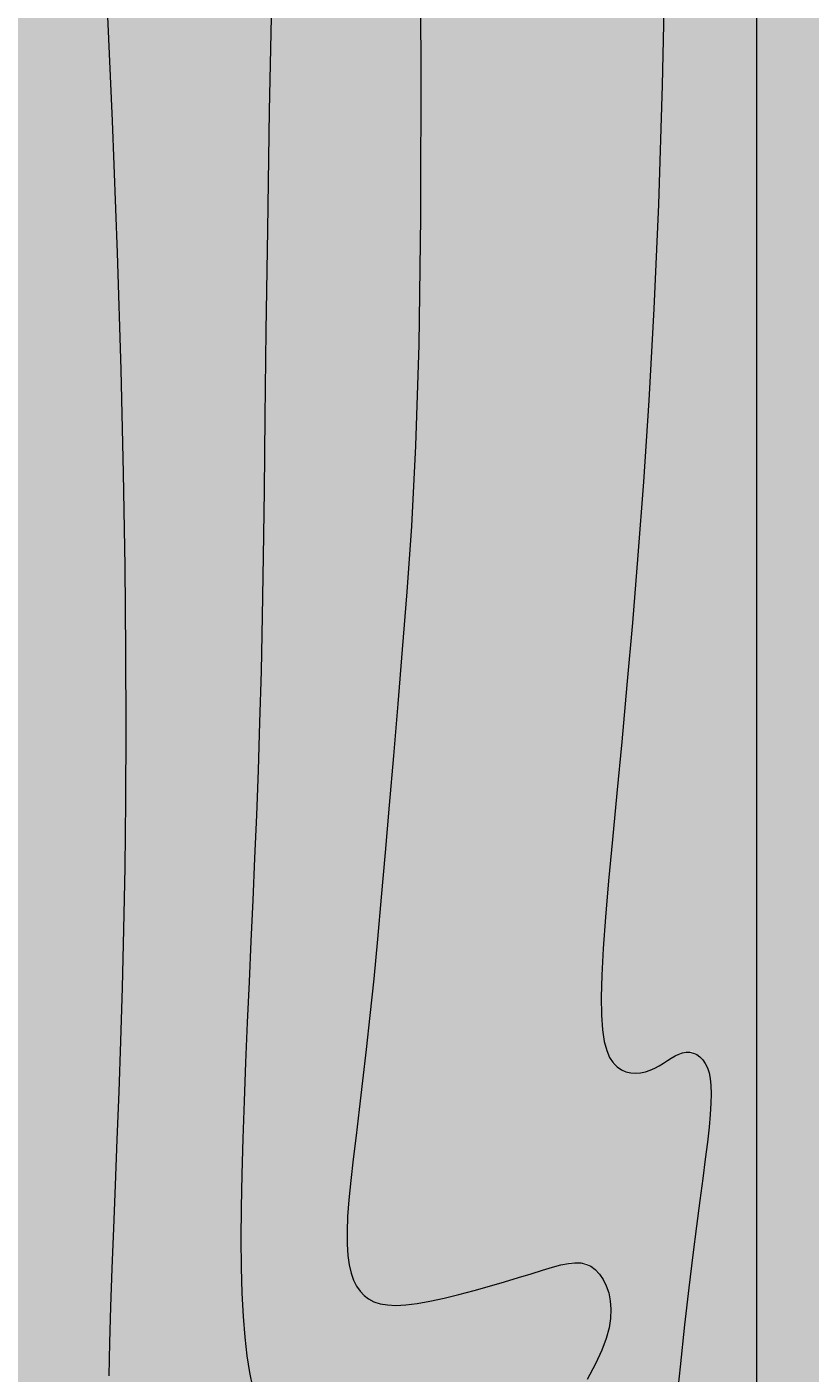
# Model space of a CAD drawing. Units: millimetres. Extents: x -229 to 16545, y -10488 to 4272.
# Tile 17 of 29: x 12216 to 12629, y -3417 to -2708. Entities that reach past the tile are written whole.
import ezdxf

# ---------------------------------------------------------------- set-up
doc = ezdxf.new("R2010")
doc.units = ezdxf.units.MM
for name, color, linetype, lineweight in [('A-ANNO-DIMS', 2, 'Continuous', 18), ('A-FURN', 8, 'Continuous', 18), ('A-FURN-PATT', 252, 'Continuous', 13)]:
    doc.layers.add(name, color=color, linetype=linetype, lineweight=lineweight)
doc.layers.add('A-FLOR-PATT', color=254, linetype='Continuous', lineweight=13, true_color=0xfeeab9)
doc.styles.get("Standard").update_dxf_attribs({"font": 'arial.ttf'})
doc.dimstyles.get("Standard").update_dxf_attribs({"dimtxt": 0.18, "dimasz": 0.18, "dimexe": 0.18, "dimexo": 0.0625, "dimgap": 0.09, "dimtad": 0, "dimtih": 1, "dimtoh": 1, "dimdec": 4, "dimzin": 0, "dimdsep": 46, "dimtxsty": 'Standard', "dimcen": 0.09, "dimadec": 0, "dimazin": 0, "dimtfac": 1, "dimtdec": 4, "dimtofl": 0, "dimtmove": 0, "dimatfit": 3, "dimfxl": 1, "dimtolj": 1, "dimtzin": 0, "dimarcsym": 0})

# ---------------------------------------------------------------- blocks, each defined once
blk = doc.blocks.new('Table - Rectangular Woodgrain 60 x 30 in.')
blk.add_line((60, 0), (0, 0))
for points in [[(9.0302, -2.4688), (12.709, -2.5477), (15.9167, -2.65), (18.7181, -2.7711), (21.1781, -2.9063), (23.3616, -3.0508), (25.3333, -3.2), (27.1477, -3.3495), (28.8172, -3.4958), (30.3437, -3.636), (31.7291, -3.7667), (32.9756, -3.8849), (34.0849, -3.9875), (35.059, -4.0714), (35.9, -4.1334), (36.6114, -4.1711), (37.2041, -4.1854), (37.6906, -4.1779), (38.0833, -4.15), (38.3948, -4.1034), (38.6375, -4.0396), (38.8239, -3.9602), (38.9666, -3.8667), (39.0764, -3.7608), (39.1573, -3.6448), (39.2116, -3.521), (39.2416, -3.3917), (39.2498, -3.2593), (39.2385, -3.1261), (39.21, -2.9944), (39.1666, -2.8667), (39.111, -2.7447), (39.0468, -2.6281), (38.978, -2.5163), (38.9083, -2.4083), (38.8418, -2.3035), (38.7823, -2.201), (38.7337, -2.1001), (38.7, -2), (38.6844, -1.9003), (38.6875, -1.8021), (38.7094, -1.707), (38.75, -1.6167), (38.8094, -1.5326), (38.8875, -1.4563), (38.9844, -1.3893), (39.1, -1.3333), (39.2351, -1.2896), (39.3937, -1.2583), (39.5804, -1.2396), (39.8, -1.2333), (40.057, -1.2396), (40.3562, -1.2583), (40.7023, -1.2896), (41.1, -1.3333), (41.5547, -1.3895), (42.0755, -1.4573), (42.6721, -1.5361), (43.3542, -1.625), (44.1316, -1.7233), (45.014, -1.8302), (46.0114, -1.9449), (47.1333, -2.0667), (48.3862, -2.1947)], [(6.5759, -9.0858), (11.9385, -9.0365), (16.2527, -9.0418), (19.6833, -9.0917), (22.3952, -9.1759), (24.5531, -9.2844), (26.322, -9.4069), (27.8666, -9.5333), (29.3241, -9.6553), (30.7203, -9.7719), (32.0532, -9.8837), (33.3208, -9.9917), (34.5213, -10.0965), (35.6526, -10.199), (36.7128, -10.2999), (37.7, -10.4), (38.6129, -10.4996), (39.4531, -10.5969), (40.223, -10.6895), (40.925, -10.775), (41.5613, -10.8512), (42.1344, -10.9156), (42.6465, -10.966), (43.1, -11), (43.4976, -11.0158), (43.8437, -11.0136), (44.143, -10.9942), (44.4, -10.9583), (44.6195, -10.9069), (44.8062, -10.8406), (44.9648, -10.7603), (45.1, -10.6667), (45.2155, -10.5598), (45.3114, -10.4365), (45.3871, -10.2929), (45.4416, -10.125), (45.4743, -9.929), (45.4844, -9.7011), (45.4709, -9.4371), (45.4333, -9.1333), (45.3716, -8.7883), (45.2896, -8.4104), (45.1919, -8.0107), (45.0833, -7.6), (44.9685, -7.1893), (44.8521, -6.7896), (44.7388, -6.4117), (44.6333, -6.0667), (44.54, -5.7628), (44.4614, -5.4979), (44.4001, -5.2675), (44.3583, -5.0667), (44.3384, -4.8909), (44.3427, -4.7354), (44.3736, -4.5956), (44.4333, -4.4667), (44.5236, -4.3453), (44.6427, -4.2333), (44.7884, -4.1339), (44.9583, -4.05), (45.1501, -3.9849), (45.3614, -3.9417), (45.59, -3.9234), (45.8333, -3.9333), (46.0915, -3.9749), (46.3734, -4.0531), (46.6906, -4.1736), (47.0542, -4.3417), (47.4756, -4.5629)], [(9.6213, -13.0323), (13.3963, -13.1059), (16.5958, -13.1583), (19.3063, -13.1952), (21.614, -13.2219), (23.6054, -13.2439), (25.3666, -13.2667), (26.9728, -13.2947), (28.4531, -13.3281), (29.8256, -13.3663), (31.1083, -13.4083), (32.3191, -13.4535), (33.476, -13.501), (34.597, -13.5501), (35.7, -13.6), (36.7984, -13.6497), (37.8875, -13.6979), (38.9578, -13.743), (40, -13.7833), (41.0047, -13.8174), (41.9625, -13.8438), (42.864, -13.8607), (43.7, -13.8667), (44.4631, -13.8604), (45.1552, -13.8417), (45.7801, -13.8104), (46.3416, -13.7667), (46.8439, -13.7104), (47.2906, -13.6417), (47.6858, -13.5604)], [(9.6609, -17.5057), (13.6705, -17.3303), (17.2125, -17.1958), (20.3467, -17.0973), (23.1328, -17.0297), (25.6307, -16.9878), (27.9, -16.9667), (29.9928, -16.9617), (31.9302, -16.9703), (33.7254, -16.9907), (35.3917, -17.0208), (36.9423, -17.0588), (38.3906, -17.1026), (39.7499, -17.1503), (41.0333, -17.2), (42.2519, -17.2496), (43.4073, -17.2969), (44.4986, -17.3395), (45.525, -17.375), (46.4858, -17.4012), (47.3802, -17.4156)]]:
    blk.add_lwpolyline(points)
blk = doc.blocks.new('*D101')
at = {"layer": 'A-ANNO-DIMS', "color": 0, "lineweight": -2, "transparency": 16777216}
for p, q in [((10907.81, -3049.71), (10907.99, -3049.71)), ((10907.9, -3049.8), (10907.9, -3049.62)), ((15176.85, -3049.71), (13576.18, -3049.71))]:
    blk.add_line(p, q, dxfattribs=at)
at = {"layer": 'A-ANNO-DIMS', "color": 0, "transparency": 16777216}
blk.add_solid([(13576.18, -3049.68), (13576.18, -3049.74), (13576, -3049.71)], dxfattribs=at)
at = {"layer": 'Defpoints', "color": 0, "transparency": 16777216}
for p in [(10907.9, -3049.71), (13576, -3049.71)]:
    blk.add_point(p, dxfattribs=at)
at = {"layer": 'A-ANNO-DIMS', "color": 0, "transparency": 16777216, "insert": (15177.3, -3049.71), "char_height": 0.18, "attachment_point": 5}
blk.add_mtext('\\A1;R2668', dxfattribs=at)
blk = doc.blocks.new('*D102')
at = {"layer": 'A-ANNO-DIMS', "color": 0, "lineweight": -2, "transparency": 16777216}
for p, q in [((11192.83, -3049.71), (11193.01, -3049.71)), ((11192.92, -3049.8), (11192.92, -3049.62)), ((15217.18, -3049.71), (13708.26, -3049.71))]:
    blk.add_line(p, q, dxfattribs=at)
at = {"layer": 'A-ANNO-DIMS', "color": 0, "transparency": 16777216}
blk.add_solid([(13708.26, -3049.68), (13708.26, -3049.74), (13708.08, -3049.71)], dxfattribs=at)
at = {"layer": 'Defpoints', "color": 0, "transparency": 16777216}
for p in [(11192.92, -3049.71), (13708.08, -3049.71)]:
    blk.add_point(p, dxfattribs=at)
at = {"layer": 'A-ANNO-DIMS', "color": 0, "transparency": 16777216, "insert": (15217.62, -3049.71), "char_height": 0.18, "attachment_point": 5}
blk.add_mtext('\\A1;R2515', dxfattribs=at)

msp = doc.modelspace()

# ---------------------------------------------------------------- hatches: boundary and pattern name
at = {"layer": 'A-FLOR-PATT', "transparency": 33554592}
h = msp.add_hatch(color=256, dxfattribs=at)
h.dxf.hatch_style = 1
h.paths.add_polyline_path([(7975.933, -5325.772), (7943.121, -5325.772), (7943.121, -4576.49, 0.4014527), (7225.933, -5325.772, 0.4014527), (6508.746, -4576.49), (6508.746, -5325.772), (6475.933, -5325.772), (6475.933, -5438.272), (5975.933, -5438.272), (5975.933, -7267.724), (5975.933, -7438.272), (6478.619, -7438.272), (6463.448, -7355.919), (6464.88, -7356.837), (6463.849, -7358.097), (6478.619, -7438.272), (6610.327, -7438.272), (6632.656, -7409.564), (6632.525, -7406.967), (6634.208, -7407.569), (6619.273, -7426.77), (6654.466, -7438.272), (7610.517, -7438.272), (7607.41, -7421.409), (7608.842, -7422.327), (7607.812, -7423.587), (7610.517, -7438.272), (7975.933, -7438.272)])
h.paths.add_polyline_path([(13785.933, -1208.272), (9555.933, -1208.272), (9555.933, -961.785), (9705.933, -961.785), (9705.933, -918.035), (10704.976, -918.035, 0.4014527), (9705.933, 38.215), (9555.933, 38.215), (9555.933, 2021.728), (5975.933, 2021.728), (5975.933, 755.492), (5745.933, 755.492), (5745.933, 1427.266), (2918.813, 1427.266), (2918.813, -492.942), (5013.319, -492.942), (5013.319, -978.272), (5745.933, -978.272), (5745.933, -397.513), (5975.933, -397.513), (5975.933, -1208.272), (4560.933, -1208.272), (4560.933, -1265.772), (4448.433, -1265.772), (4448.433, -1298.585), (4445.933, -1298.585), (3699.151, -1298.585, 0.4014527), (4448.433, -2015.772), (4560.933, -2015.772), (4560.933, -2384.177), (5745.933, -2384.177), (5799.402, -2384.177), (5799.402, -4518.272), (5975.933, -4518.272), (5975.933, -5208.272), (6475.933, -5208.272), (6475.933, -4575.772), (6508.746, -4575.772), (6508.746, -4576.49, -0.3564726), (7216.672, -5208.272), (7235.194, -5208.272, -0.3564726), (7943.121, -4576.49), (7943.121, -4575.772), (7975.933, -4575.772), (7975.933, -5208.272), (11176.247, -5208.272), (11159.44, -5191.465), (10520.768, -5191.465), (10520.768, -4888.936), (10571.19, -4888.936), (10571.19, -4872.129), (10772.876, -4872.129), (10772.876, -4888.936), (10789.683, -4888.936), (10789.683, -4872.129), (10991.368, -4872.129), (10991.368, -4888.936), (11041.79, -4888.936), (11041.79, -4872.129), (11058.597, -4872.129, -0.0909091), (11428.354, -4872.129), (11445.162, -4872.129), (11445.162, -4888.936), (11529.197, -4888.936), (11529.197, -5191.465), (11327.512, -5191.465), (11310.704, -5208.272), (13785.933, -5208.272)])
h.paths.add_polyline_path([(11047.216, -1630.944, -1), (11402.816, -1630.944, -1)], flags=16)
h.paths.add_polyline_path([(11148.816, -1630.944), (11225.016, -1554.744), (11301.216, -1630.944), (11225.016, -1707.144)], flags=0)
h.paths.add_polyline_path([(11199.616, -1630.944, -1), (11250.416, -1630.944, -1)], flags=0)
h.paths.add_polyline_path([(11588.751, -2096.259), (11588.751, -1543.254, -0.266667), (12864.918, -1543.254), (12864.918, -2096.259), (12737.302, -2096.259), (12737.302, -2063.121), (11716.368, -2063.121), (11716.368, -2096.259)], flags=16)
h.paths.add_polyline_path([(12012.696, -2489.42), (12600.997, -2489.42), (12600.997, -3666.022), (12012.696, -3666.022)], flags=16)
h.paths.add_polyline_path([(12176.41, -3599.403), (12174.938, -3609.076), (12173.789, -3618.819), (12173.09, -3628.559), (12172.973, -3638.221), (12173.89, -3652.852), (12175.008, -3657.025), (12172.909, -3643.473), (12173.142, -3624.297), (12175.386, -3605.273)], flags=0)
h.paths.add_polyline_path([(8026.289, -286.944), (7737.703, -287.19), (7734.87, -269.156), (8029.092, -268.905)], flags=16)
h.paths.add_polyline_path([(7733.453, -260.139), (7710.784, -115.865), (7557.191, -115.996), (7556.999, 109.744), (7412.687, 132.166), (7412.433, 429.206), (7556.707, 451.876), (7556.568, 614.769), (7412.256, 637.19), (7412.003, 934.231), (7556.276, 956.9), (7556.084, 1182.639), (7709.677, 1182.77), (7732.099, 1327.082), (8029.14, 1327.335), (8051.808, 1183.062), (8205.401, 1183.192), (8205.594, 957.454), (8349.906, 935.031), (8350.159, 637.99), (8205.885, 615.322), (8206.024, 452.43), (8350.336, 430.006), (8350.59, 132.965), (8206.316, 110.298), (8206.509, -115.442), (8052.916, -115.573), (8030.493, -259.885)], flags=16)
h.paths.add_polyline_path([(12261.416, -3475.554), (12262.632, -3486.776), (12264.032, -3497.007), (12265.554, -3506.365), (12267.136, -3514.968), (12268.719, -3522.935), (12271.304, -3535.59), (12273.606, -3548.078), (12275.271, -3561.064), (12275.93, -3574.938), (12275.325, -3590.3), (12273.425, -3607.964), (12270.795, -3625.658), (12268.066, -3641.063), (12266.318, -3649.679), (12265.456, -3653.626), (12263.984, -3659.846), (12264.032, -3659.566), (12264.342, -3658.241), (12264.807, -3656.37), (12265.456, -3653.626), (12266.318, -3649.679), (12267.409, -3644.302), (12268.668, -3637.664), (12270.019, -3630.037), (12271.384, -3621.695), (12272.69, -3612.908), (12273.857, -3603.948), (12274.81, -3595.088), (12275.47, -3586.601), (12275.782, -3578.689), (12275.757, -3571.292), (12275.423, -3564.275), (12274.816, -3557.512), (12273.964, -3550.872), (12272.896, -3544.224), (12271.645, -3537.439), (12270.24, -3530.385), (12267.543, -3517.181), (12264.612, -3501.247), (12261.849, -3481.059)], flags=0)
h.paths.add_polyline_path([(12332.136, -3408.03), (12333.483, -3416.79), (12335.077, -3424.54), (12336.915, -3431.355), (12338.991, -3437.32), (12341.266, -3442.55), (12343.694, -3447.166), (12346.229, -3451.292), (12348.826, -3455.051), (12351.438, -3458.563), (12357.476, -3466.491), (12363.61, -3476.575), (12368.309, -3489.762), (12369.929, -3503.427), (12369.842, -3516.511), (12368.43, -3530.867), (12365.816, -3545.835), (12362.382, -3559.786), (12360.968, -3564.487), (12363.063, -3557.021), (12364.898, -3549.566), (12366.473, -3542.077), (12367.773, -3534.631), (12368.781, -3527.301), (12369.483, -3520.162), (12369.863, -3513.291), (12369.906, -3506.759), (12369.599, -3500.643), (12368.93, -3494.999), (12367.924, -3489.796), (12366.61, -3484.994), (12365.024, -3480.542), (12363.19, -3476.399), (12361.141, -3472.516), (12358.909, -3468.847), (12356.525, -3465.347), (12354.02, -3461.954), (12351.438, -3458.563), (12345.462, -3450.529), (12339.923, -3439.996), (12335.85, -3428.296), (12332.68, -3412.888)], flags=0)
h.paths.add_polyline_path([(12385.287, -3334.612), (12384.977, -3342.409), (12385.02, -3349.196), (12385.4, -3355.066), (12386.104, -3360.105), (12387.112, -3364.41), (12388.412, -3368.071), (12389.987, -3371.181), (12391.823, -3373.832), (12393.919, -3376.097), (12396.337, -3377.978), (12399.153, -3379.462), (12402.445, -3380.531), (12406.289, -3381.172), (12410.758, -3381.371), (12415.935, -3381.106), (12421.893, -3380.368), (12428.658, -3379.159), (12436.069, -3377.55), (12443.907, -3375.635), (12451.961, -3373.505), (12460.015, -3371.254), (12467.853, -3368.971), (12475.263, -3366.749), (12482.029, -3364.68), (12491.877, -3361.657), (12497.701, -3360.107), (12501.639, -3359.288), (12510.135, -3358.326), (12519.662, -3365.412), (12524.243, -3378.911), (12523.764, -3390.7), (12520.746, -3401.577), (12514.248, -3415.634), (12511.518, -3420.418), (12515.856, -3412.154), (12519.153, -3405.024), (12521.516, -3398.804), (12523.049, -3393.276), (12523.865, -3388.212), (12524.059, -3383.441), (12523.7, -3378.958), (12522.853, -3374.815), (12521.576, -3371.054), (12519.931, -3367.722), (12517.982, -3364.865), (12515.786, -3362.529), (12513.405, -3360.758), (12510.877, -3359.588), (12508.136, -3358.982), (12505.086, -3358.897), (12501.639, -3359.288), (12497.701, -3360.107), (12493.183, -3361.309), (12487.988, -3362.851), (12476.403, -3366.408), (12463.335, -3370.326), (12447.372, -3374.788), (12431.759, -3378.604), (12418.504, -3380.974), (12405.811, -3381.624), (12394.725, -3378.025), (12388.039, -3368.367), (12385.583, -3357.877), (12384.826, -3346.204), (12385.428, -3331.059), (12385.953, -3325.719)], flags=0)
h.paths.add_polyline_path([(7880.016, 1173.969), (7880.373, 1175.495), (7880.433, 1175.851), (7879.484, 1171.818)], flags=0)
h.paths.add_polyline_path([(7802.33, 874.962), (7800.771, 885.032), (7798.932, 893.941), (7796.811, 901.774), (7794.419, 908.63), (7791.798, 914.639), (7789.002, 919.945), (7786.083, 924.686), (7783.093, 929.005), (7780.087, 933.043), (7774.996, 939.717), (7768.406, 949.37), (7762.174, 963.427), (7759.342, 978.002), (7758.629, 991.888), (7759.492, 1007.928), (7761.801, 1025.496), (7765.392, 1044.035), (7766.625, 1049.048), (7764.522, 1039.543), (7762.719, 1030.232), (7761.232, 1021.168), (7760.08, 1012.405), (7759.28, 1003.994), (7758.849, 995.988), (7758.806, 988.44), (7759.167, 981.404), (7759.942, 974.914), (7761.104, 968.936), (7762.617, 963.414), (7764.448, 958.299), (7766.559, 953.535), (7768.918, 949.073), (7771.487, 944.856), (7774.232, 940.835), (7777.115, 936.938), (7782.377, 930.041), (7787.845, 922.139), (7793.348, 911.698), (7798.042, 898.247), (7801.702, 880.527)], flags=0)
h.paths.add_polyline_path([(12519.068, -3228.534), (12519.615, -3236.235), (12520.529, -3242.343), (12521.78, -3247.103), (12523.337, -3250.758), (12525.171, -3253.556), (12527.248, -3255.709), (12529.522, -3257.296), (12531.95, -3258.361), (12534.486, -3258.949), (12537.082, -3259.11), (12539.694, -3258.888), (12542.277, -3258.329), (12544.781, -3257.478), (12547.173, -3256.388), (12549.46, -3255.129), (12550.455, -3254.517), (12555.825, -3251.109), (12557.835, -3249.942), (12565.181, -3246.404), (12574.565, -3253.032), (12576.931, -3265.022), (12576.627, -3277.425), (12575.416, -3290.819), (12574.851, -3295.392), (12575.708, -3287.593), (12576.322, -3280.806), (12576.688, -3274.939), (12576.812, -3269.899), (12576.688, -3265.593), (12576.322, -3261.932), (12575.708, -3258.822), (12574.851, -3256.172), (12573.753, -3253.905), (12572.439, -3252.005), (12570.943, -3250.474), (12569.293, -3249.309), (12567.523, -3248.513), (12565.658, -3248.083), (12563.732, -3248.022), (12561.777, -3248.328), (12559.814, -3248.989), (12557.835, -3249.942), (12555.825, -3251.109), (12553.77, -3252.413), (12551.652, -3253.78), (12549.46, -3255.129), (12543.167, -3258.594), (12532.661, -3259.485), (12524.685, -3253.923), (12520.949, -3245.152), (12519.138, -3233.042)], flags=0)
h.paths.add_polyline_path([(7741.293, 790.501), (7741.641, 799.467), (7741.584, 807.269), (7741.141, 814.015), (7740.329, 819.809), (7739.165, 824.757), (7737.667, 828.966), (7735.853, 832.541), (7733.74, 835.586), (7731.348, 838.188), (7728.71, 840.348), (7725.861, 842.052), (7722.836, 843.28), (7719.671, 844.015), (7716.4, 844.237), (7713.06, 843.932), (7709.684, 843.081), (7706.304, 841.686), (7702.923, 839.834), (7699.543, 837.629), (7696.164, 835.178), (7692.784, 832.585), (7684.718, 826.315), (7675.609, 820.63), (7664.001, 817.274), (7654.105, 821.884), (7647.171, 832.02), (7644.191, 846.522), (7646.321, 860.288), (7647.49, 864.223), (7645.946, 857.865), (7645.046, 852.044), (7644.827, 846.557), (7645.243, 841.404), (7646.221, 836.642), (7647.693, 832.318), (7649.587, 828.489), (7651.832, 825.206), (7654.359, 822.523), (7657.097, 820.49), (7659.984, 819.145), (7662.993, 818.452), (7666.108, 818.357), (7669.311, 818.809), (7672.583, 819.755), (7675.908, 821.139), (7679.268, 822.913), (7682.645, 825.021), (7686.025, 827.401), (7689.404, 829.958), (7692.784, 832.585), (7700.505, 838.509), (7709.871, 843.64), (7721.436, 844.698), (7733.277, 837.617), (7739.571, 825.214), (7741.557, 811.049), (7741.669, 795.575)], flags=0)
h.paths.add_polyline_path([(8377.641, 137.216), (8359.607, 134.382), (8359.356, 428.605), (8377.395, 425.802)], flags=16)
h.paths.add_polyline_path([(7650.715, 668.465), (7650.08, 677.319), (7649.023, 684.34), (7647.579, 689.811), (7645.785, 694.012), (7643.675, 697.228), (7641.286, 699.7), (7638.669, 701.521), (7635.876, 702.744), (7632.96, 703.419), (7629.974, 703.601), (7626.971, 703.344), (7624.004, 702.697), (7621.125, 701.717), (7618.375, 700.462), (7615.749, 699.013), (7614.561, 698.279), (7608.435, 694.382), (7606.125, 693.04), (7598.981, 689.594), (7589.669, 693.773), (7585.26, 702.856), (7584.221, 713.11), (7584.49, 724.584), (7585.863, 739.937), (7586.518, 745.277), (7585.539, 736.31), (7584.841, 728.507), (7584.424, 721.761), (7584.288, 715.966), (7584.433, 711.016), (7584.86, 706.807), (7585.567, 703.231), (7586.556, 700.186), (7587.821, 697.58), (7589.332, 695.397), (7591.053, 693.637), (7592.951, 692.3), (7594.989, 691.385), (7597.132, 690.895), (7599.346, 690.826), (7601.594, 691.18), (7603.851, 691.943), (7606.125, 693.04), (7608.435, 694.382), (7610.797, 695.885), (7613.229, 697.458), (7620.475, 701.929), (7632.001, 704.44), (7643.476, 699.417), (7648.536, 687.571), (7650.63, 673.661)], flags=0)
h.paths.add_polyline_path([(7385.628, 136.37), (7385.382, 424.956), (7403.416, 427.789), (7403.667, 133.567)], flags=16)
h.paths.add_polyline_path([(12993.884, -2257.186), (12959.588, -2257.186), (12959.588, -2125.099), (13531.966, -2125.099, -0.1904762), (13531.966, -3974.321), (12959.588, -3974.321), (12959.588, -3842.233), (12993.884, -3842.233)], flags=16)
h.paths.add_polyline_path([(13413.486, -3313.884), (13413.486, -2785.535), (13562.885, -2785.535, -0.0496282), (13562.885, -3313.884)], flags=0)
h.paths.add_polyline_path([(8377.21, 642.241), (8359.176, 639.407), (8358.925, 933.629), (8376.964, 930.826)], flags=16)
h.paths.add_polyline_path([(13086.058, -1864.83), (13086.058, -1449.84), (13501.048, -1449.84), (13501.048, -1864.83)], flags=16)
h.paths.add_polyline_path([(13305.814, -1862.197), (13302.103, -1859.624), (13298.088, -1857.068), (13293.799, -1854.536), (13289.262, -1852.031), (13284.504, -1849.559), (13279.554, -1847.125), (13274.439, -1844.735), (13269.17, -1842.389), (13263.701, -1840.081), (13257.97, -1837.797), (13251.914, -1835.525), (13245.472, -1833.252), (13238.582, -1830.968), (13231.18, -1828.66), (13223.206, -1826.315), (13209.182, -1822.458), (13204.584, -1821.48), (13217.962, -1824.773), (13235.072, -1829.804), (13248.777, -1834.349), (13260.829, -1838.869), (13274.479, -1844.63), (13289.675, -1852.101), (13302.553, -1859.704)], flags=0)
h.paths.add_polyline_path([(13428.104, -1820.994), (13419.007, -1818.141), (13409.95, -1815.4), (13400.766, -1812.747), (13391.271, -1810.151), (13376.087, -1806.251), (13370.618, -1805.019), (13386.304, -1808.794), (13405.087, -1813.928), (13423.014, -1819.354)], flags=0)
h.paths.add_polyline_path([(7385.197, 641.395), (7384.951, 929.98), (7402.986, 932.814), (7403.236, 638.592)], flags=16)
h.paths.add_polyline_path([(13262.537, -1725.526), (13253.246, -1724.74), (13244.516, -1724.117), (13235.94, -1723.625), (13223.267, -1723.062), (13217.598, -1722.912), (13231.966, -1723.397), (13248.733, -1724.359), (13266.899, -1725.895), (13272.802, -1726.502)], flags=0)
h.paths.add_polyline_path([(13191.893, -1641.137), (13208.675, -1640.506), (13214.057, -1640.258), (13197.763, -1640.936)], flags=0)
h.paths.add_polyline_path([(13097.524, -1608.457), (13114.284, -1609.031), (13120.126, -1609.105), (13103.045, -1608.71)], flags=0)
h.paths.add_polyline_path([(13465.328, -1521.577), (13473.906, -1517.015), (13481.761, -1511.636), (13492.562, -1502.076), (13495.327, -1497.933), (13485.818, -1508.858), (13470.208, -1519.547)], flags=0)
h.paths.add_polyline_path([(13175.015, -1500.891), (13184.046, -1501.807), (13192.721, -1502.52), (13201.114, -1503.034), (13209.273, -1503.351), (13217.244, -1503.476), (13225.078, -1503.41), (13232.821, -1503.16), (13240.524, -1502.728), (13248.233, -1502.117), (13255.993, -1501.322), (13263.825, -1500.293), (13271.746, -1498.974), (13279.775, -1497.305), (13287.928, -1495.229), (13296.222, -1492.688), (13304.675, -1489.622), (13313.304, -1485.975), (13322.089, -1481.727), (13330.859, -1477.028), (13339.408, -1472.063), (13347.526, -1467.02), (13355.006, -1462.087), (13364.86, -1455.202), (13367.224, -1453.299), (13358.544, -1459.754), (13343.348, -1469.775), (13326.143, -1479.767), (13309.023, -1488.045), (13292.249, -1494.129), (13276.009, -1498.264), (13260.299, -1500.88), (13244.401, -1502.51), (13228.945, -1503.378), (13213.316, -1503.508), (13197.047, -1502.876), (13180.088, -1501.481)], flags=0)
h.paths.add_polyline_path([(7733.501, 1336.101), (7736.303, 1354.14), (8024.889, 1354.386), (8027.723, 1336.352)], flags=16)
at = {"layer": 'A-FURN-PATT', "transparency": 33554569}
h = msp.add_hatch(color=256, dxfattribs=at)
h.dxf.hatch_style = 1
h.paths.add_polyline_path([(12600.997, -2489.42), (12553.933, -2489.42), (12553.58, -2583.852), (12552.584, -2666.503), (12551.036, -2738.644), (12549.03, -2801.547), (12546.656, -2856.483), (12544.004, -2904.723), (12541.171, -2947.542), (12538.245, -2986.207), (12535.313, -3021.787), (12532.444, -3054.526), (12529.695, -3084.461), (12527.132, -3111.629), (12524.814, -3136.073), (12522.802, -3157.826), (12521.157, -3176.928), (12519.941, -3193.42), (12519.202, -3207.371), (12518.921, -3218.994), (12519.068, -3228.534), (12519.615, -3236.235), (12520.529, -3242.343), (12521.78, -3247.103), (12523.337, -3250.758), (12525.171, -3253.556), (12527.248, -3255.709), (12529.522, -3257.296), (12531.95, -3258.361), (12534.486, -3258.949), (12537.082, -3259.11), (12539.694, -3258.888), (12542.277, -3258.329), (12544.781, -3257.478), (12547.173, -3256.388), (12549.46, -3255.129), (12551.652, -3253.78), (12559.563, -3248.675), (12566.794, -3247.543), (12572.687, -3251.706), (12575.978, -3258.498), (12576.872, -3267.431), (12576.627, -3277.425), (12575.708, -3287.593), (12574.851, -3295.392), (12573.749, -3304.309), (12572.419, -3314.522), (12570.874, -3326.221), (12569.131, -3339.597), (12567.203, -3354.842), (12565.107, -3372.146), (12562.857, -3391.705), (12560.469, -3413.705), (12557.959, -3438.275), (12555.343, -3465.264), (12552.633, -3494.46), (12549.848, -3525.645), (12547.001, -3558.61), (12544.106, -3593.137), (12541.184, -3629.012), (12538.245, -3666.022), (12600.997, -3666.022)])
h.paths.add_polyline_path([(12544.004, -2904.723), (12546.656, -2856.483), (12549.03, -2801.547), (12551.036, -2738.644), (12552.584, -2666.503), (12553.58, -2583.852), (12553.933, -2489.42), (12420.585, -2489.42), (12422.824, -2618.374), (12423.791, -2723.534), (12423.687, -2808.136), (12422.708, -2875.41), (12421.057, -2928.591), (12418.93, -2970.907), (12416.527, -3005.595), (12414.049, -3035.885), (12411.656, -3064.467), (12409.37, -3091.846), (12407.177, -3117.984), (12405.059, -3142.842), (12403.004, -3166.384), (12400.994, -3188.569), (12399.016, -3209.359), (12397.053, -3228.718), (12395.1, -3246.62), (12393.191, -3263.097), (12391.376, -3278.194), (12389.699, -3291.961), (12388.205, -3304.438), (12386.942, -3315.677), (12385.953, -3325.719), (12385.287, -3334.612), (12384.977, -3342.409), (12385.02, -3349.196), (12385.4, -3355.066), (12386.104, -3360.105), (12387.112, -3364.41), (12388.412, -3368.071), (12389.987, -3371.181), (12391.823, -3373.832), (12393.919, -3376.097), (12396.337, -3377.978), (12399.153, -3379.462), (12402.445, -3380.531), (12406.289, -3381.172), (12410.758, -3381.371), (12415.935, -3381.106), (12421.893, -3380.368), (12428.658, -3379.159), (12436.069, -3377.55), (12443.907, -3375.635), (12451.961, -3373.505), (12460.015, -3371.254), (12467.853, -3368.971), (12475.263, -3366.749), (12482.029, -3364.68), (12491.877, -3361.657), (12502.516, -3358.826), (12511.128, -3359.064), (12517.01, -3363.44), (12520.955, -3369.223), (12523.527, -3376.802), (12524.25, -3385.824), (12522.632, -3395.865), (12519.153, -3405.024), (12515.856, -3412.154), (12511.518, -3420.418), (12506.031, -3430.037), (12499.288, -3441.236), (12491.181, -3454.234), (12481.682, -3469.286), (12471.081, -3486.774), (12459.744, -3507.112), (12448.039, -3530.713), (12436.334, -3557.99), (12424.997, -3589.358), (12414.396, -3625.231), (12404.897, -3666.022), (12538.245, -3666.022), (12541.184, -3629.012), (12544.106, -3593.137), (12547.001, -3558.61), (12549.848, -3525.645), (12552.633, -3494.46), (12555.343, -3465.264), (12557.959, -3438.275), (12560.469, -3413.705), (12562.857, -3391.705), (12565.107, -3372.146), (12567.203, -3354.842), (12569.131, -3339.597), (12570.874, -3326.221), (12572.419, -3314.522), (12573.749, -3304.309), (12574.851, -3295.392), (12575.708, -3287.593), (12576.322, -3280.806), (12576.688, -3274.939), (12576.812, -3269.899), (12576.688, -3265.593), (12576.322, -3261.932), (12575.708, -3258.822), (12574.851, -3256.172), (12573.753, -3253.905), (12572.439, -3252.005), (12570.943, -3250.474), (12569.293, -3249.309), (12567.523, -3248.513), (12565.658, -3248.083), (12563.732, -3248.022), (12561.777, -3248.328), (12559.814, -3248.989), (12557.835, -3249.942), (12555.825, -3251.109), (12553.77, -3252.413), (12547.19, -3256.659), (12539.533, -3259.262), (12531.64, -3258.773), (12524.685, -3253.923), (12520.949, -3245.152), (12519.615, -3236.235), (12519.068, -3228.534), (12518.921, -3218.994), (12519.202, -3207.371), (12519.941, -3193.42), (12521.157, -3176.928), (12522.802, -3157.826), (12524.814, -3136.073), (12527.132, -3111.629), (12529.695, -3084.461), (12532.444, -3054.526), (12535.313, -3021.787), (12538.245, -2986.207), (12541.171, -2947.542)])
h.paths.add_polyline_path([(12418.93, -2970.907), (12421.057, -2928.591), (12422.708, -2875.41), (12423.687, -2808.136), (12423.791, -2723.534), (12422.824, -2618.374), (12420.585, -2489.42), (12349.989, -2489.42), (12347.396, -2591.092), (12345.433, -2678.094), (12343.99, -2752.122), (12342.962, -2814.864), (12342.239, -2868.017), (12341.715, -2913.271), (12341.284, -2952.323), (12340.837, -2986.86), (12340.288, -3018.358), (12339.633, -3047.386), (12338.883, -3074.301), (12338.06, -3099.455), (12337.173, -3123.199), (12336.242, -3145.885), (12335.279, -3167.868), (12334.301, -3189.498), (12333.326, -3211.038), (12332.381, -3232.395), (12331.496, -3253.384), (12330.706, -3273.821), (12330.037, -3293.523), (12329.52, -3312.306), (12329.188, -3329.984), (12329.071, -3346.378), (12329.194, -3361.343), (12329.561, -3374.915), (12330.175, -3387.169), (12331.032, -3398.18), (12332.136, -3408.03), (12333.483, -3416.79), (12335.077, -3424.54), (12336.915, -3431.355), (12338.991, -3437.32), (12341.266, -3442.55), (12343.694, -3447.166), (12346.229, -3451.292), (12348.826, -3455.051), (12351.438, -3458.563), (12357.476, -3466.491), (12362.356, -3474.514), (12365.989, -3482.725), (12368.611, -3492.308), (12369.929, -3503.427), (12369.863, -3513.291), (12369.483, -3520.162), (12368.781, -3527.301), (12367.773, -3534.631), (12366.473, -3542.077), (12364.898, -3549.566), (12363.063, -3557.021), (12360.968, -3564.487), (12358.568, -3572.468), (12355.799, -3581.585), (12352.603, -3592.463), (12348.916, -3605.723), (12344.678, -3621.988), (12339.827, -3641.88), (12334.301, -3666.022), (12404.897, -3666.022), (12414.396, -3625.231), (12424.997, -3589.358), (12436.334, -3557.99), (12448.039, -3530.713), (12459.744, -3507.112), (12471.081, -3486.774), (12481.682, -3469.286), (12491.181, -3454.234), (12499.288, -3441.236), (12506.031, -3430.037), (12511.518, -3420.418), (12515.856, -3412.154), (12519.153, -3405.024), (12521.516, -3398.804), (12523.049, -3393.276), (12523.865, -3388.212), (12524.059, -3383.441), (12523.7, -3378.958), (12522.853, -3374.815), (12521.576, -3371.054), (12519.931, -3367.722), (12517.982, -3364.865), (12515.786, -3362.529), (12513.405, -3360.758), (12510.877, -3359.588), (12508.136, -3358.982), (12505.086, -3358.897), (12501.639, -3359.288), (12497.701, -3360.107), (12493.183, -3361.309), (12487.988, -3362.851), (12476.403, -3366.408), (12463.335, -3370.326), (12451.961, -3373.505), (12439.372, -3376.834), (12424.661, -3380.026), (12412.995, -3381.47), (12402.039, -3380.984), (12393.748, -3376.613), (12389.022, -3369.787), (12386.442, -3362.522), (12385.041, -3352.492), (12384.977, -3342.409), (12385.287, -3334.612), (12385.953, -3325.719), (12386.942, -3315.677), (12388.205, -3304.438), (12389.699, -3291.961), (12391.376, -3278.194), (12393.191, -3263.097), (12395.1, -3246.62), (12397.053, -3228.718), (12399.016, -3209.359), (12400.994, -3188.569), (12403.004, -3166.384), (12405.059, -3142.842), (12407.177, -3117.984), (12409.37, -3091.846), (12411.656, -3064.467), (12414.049, -3035.885), (12416.527, -3005.595)])
h.paths.add_polyline_path([(12340.837, -2986.86), (12341.284, -2952.323), (12341.715, -2913.271), (12342.239, -2868.017), (12342.962, -2814.864), (12343.99, -2752.122), (12345.433, -2678.094), (12347.396, -2591.092), (12349.989, -2489.42), (12248.016, -2489.42), (12253.364, -2589.902), (12257.71, -2678.871), (12261.149, -2757.499), (12263.787, -2826.958), (12265.718, -2888.42), (12267.044, -2943.055), (12267.866, -2992.039), (12268.279, -3036.54), (12268.378, -3077.58), (12268.209, -3115.572), (12267.809, -3150.776), (12267.219, -3183.452), (12266.473, -3213.86), (12265.614, -3242.261), (12264.679, -3268.917), (12263.704, -3294.084), (12262.732, -3317.981), (12261.804, -3340.639), (12260.969, -3362.039), (12260.273, -3382.167), (12259.759, -3401.008), (12259.477, -3418.547), (12259.469, -3434.769), (12259.782, -3449.659), (12260.445, -3463.221), (12261.416, -3475.554), (12262.632, -3486.776), (12264.032, -3497.007), (12265.554, -3506.365), (12267.136, -3514.968), (12268.719, -3522.935), (12271.304, -3535.59), (12273.606, -3548.078), (12275.271, -3561.064), (12275.757, -3571.292), (12275.782, -3578.689), (12275.47, -3586.601), (12274.81, -3595.088), (12273.857, -3603.948), (12272.69, -3612.908), (12271.384, -3621.695), (12270.019, -3630.037), (12268.066, -3641.063), (12265.651, -3652.97), (12264.342, -3658.241), (12264.032, -3659.566), (12263.842, -3660.678), (12263.746, -3661.906), (12263.708, -3663.576), (12263.704, -3666.022), (12334.301, -3666.022), (12339.827, -3641.88), (12344.678, -3621.988), (12348.916, -3605.723), (12352.603, -3592.463), (12355.799, -3581.585), (12358.568, -3572.468), (12360.968, -3564.487), (12363.063, -3557.021), (12364.898, -3549.566), (12366.473, -3542.077), (12367.773, -3534.631), (12368.781, -3527.301), (12369.483, -3520.162), (12369.863, -3513.291), (12369.906, -3506.759), (12369.599, -3500.643), (12368.93, -3494.999), (12367.924, -3489.796), (12366.61, -3484.994), (12365.024, -3480.542), (12363.19, -3476.399), (12361.141, -3472.516), (12358.909, -3468.847), (12356.525, -3465.347), (12354.02, -3461.954), (12347.609, -3453.536), (12342.257, -3444.828), (12337.759, -3434.488), (12335.077, -3424.54), (12333.483, -3416.79), (12332.136, -3408.03), (12331.032, -3398.18), (12330.175, -3387.169), (12329.561, -3374.915), (12329.194, -3361.343), (12329.071, -3346.378), (12329.188, -3329.984), (12329.52, -3312.306), (12330.037, -3293.523), (12330.706, -3273.821), (12331.496, -3253.384), (12332.381, -3232.395), (12333.326, -3211.038), (12334.301, -3189.498), (12335.279, -3167.868), (12336.242, -3145.885), (12337.173, -3123.199), (12338.06, -3099.455), (12338.883, -3074.301), (12339.633, -3047.386), (12340.288, -3018.358)])
h.paths.add_polyline_path([(12267.866, -2992.039), (12267.044, -2943.055), (12265.718, -2888.42), (12263.787, -2826.958), (12261.149, -2757.499), (12257.71, -2678.871), (12253.364, -2589.902), (12248.016, -2489.42), (12161.732, -2489.42), (12164.672, -2646.493), (12167.594, -2771.989), (12170.488, -2870.184), (12173.336, -2945.353), (12176.12, -3001.769), (12178.83, -3043.709), (12181.446, -3075.446), (12183.956, -3101.253), (12186.347, -3124.72), (12188.614, -3146.693), (12190.759, -3167.333), (12192.781, -3186.802), (12194.681, -3205.259), (12196.458, -3222.865), (12198.113, -3239.782), (12199.644, -3256.172), (12201.048, -3272.182), (12202.3, -3287.915), (12203.368, -3303.466), (12204.221, -3318.924), (12204.827, -3334.383), (12205.161, -3349.932), (12205.186, -3365.667), (12204.874, -3381.676), (12204.208, -3398.008), (12203.219, -3414.517), (12201.956, -3431.021), (12200.462, -3447.329), (12198.784, -3463.254), (12196.97, -3478.607), (12195.062, -3493.203), (12193.108, -3506.853), (12191.149, -3519.429), (12189.196, -3531.038), (12187.259, -3541.853), (12185.347, -3552.039), (12183.462, -3561.763), (12181.619, -3571.2), (12179.819, -3580.51), (12178.073, -3589.87), (12176.41, -3599.403), (12174.938, -3609.076), (12173.789, -3618.819), (12173.09, -3628.559), (12172.973, -3638.221), (12173.569, -3647.734), (12175.008, -3657.025), (12177.42, -3666.022), (12263.654, -3666.022), (12263.777, -3660.515), (12264.807, -3656.37), (12265.456, -3653.626), (12266.318, -3649.679), (12267.409, -3644.302), (12268.668, -3637.664), (12270.019, -3630.037), (12271.384, -3621.695), (12272.69, -3612.908), (12273.857, -3603.948), (12274.81, -3595.088), (12275.47, -3586.601), (12275.782, -3578.689), (12275.757, -3571.292), (12275.423, -3564.275), (12274.816, -3557.512), (12273.964, -3550.872), (12272.896, -3544.224), (12271.645, -3537.439), (12270.24, -3530.385), (12267.543, -3517.181), (12265.554, -3506.365), (12264.032, -3497.007), (12262.632, -3486.776), (12261.416, -3475.554), (12260.445, -3463.221), (12259.782, -3449.659), (12259.469, -3434.769), (12259.477, -3418.547), (12259.759, -3401.008), (12260.273, -3382.167), (12260.969, -3362.039), (12261.804, -3340.639), (12262.732, -3317.981), (12263.704, -3294.084), (12264.679, -3268.917), (12265.614, -3242.261), (12266.473, -3213.86), (12267.219, -3183.452), (12267.809, -3150.776), (12268.209, -3115.572), (12268.378, -3077.58), (12268.279, -3036.54)])
h.paths.add_polyline_path([(12178.83, -3043.709), (12176.12, -3001.769), (12173.336, -2945.353), (12170.488, -2870.184), (12167.594, -2771.989), (12164.672, -2646.493), (12161.732, -2489.42), (12106.824, -2489.42), (12109.758, -2658.763), (12112.646, -2797.349), (12115.441, -2909.171), (12118.1, -2998.218), (12120.575, -3068.485), (12122.818, -3123.958), (12124.787, -3168.631), (12126.434, -3206.494), (12127.727, -3240.902), (12128.682, -3272.678), (12129.331, -3302.001), (12129.703, -3329.057), (12129.831, -3354.028), (12129.742, -3377.101), (12129.472, -3398.457), (12129.048, -3418.282), (12128.499, -3436.761), (12127.832, -3454.092), (12127.062, -3470.478), (12126.189, -3486.119), (12125.224, -3501.217), (12124.177, -3515.972), (12123.052, -3530.585), (12121.857, -3545.257), (12120.61, -3560.145), (12119.355, -3575.225), (12118.147, -3590.433), (12117.037, -3605.699), (12116.082, -3620.96), (12115.331, -3636.144), (12114.843, -3651.187), (12114.668, -3666.022), (12177.42, -3666.022), (12175.008, -3657.025), (12173.569, -3647.734), (12172.973, -3638.221), (12173.09, -3628.559), (12173.789, -3618.819), (12174.938, -3609.076), (12176.41, -3599.403), (12178.073, -3589.87), (12179.819, -3580.51), (12181.619, -3571.2), (12183.462, -3561.763), (12185.347, -3552.039), (12187.259, -3541.853), (12189.196, -3531.038), (12191.149, -3519.429), (12193.108, -3506.853), (12195.062, -3493.203), (12196.97, -3478.607), (12198.784, -3463.254), (12200.462, -3447.329), (12201.956, -3431.021), (12203.219, -3414.517), (12204.208, -3398.008), (12204.874, -3381.676), (12205.186, -3365.667), (12205.161, -3349.932), (12204.827, -3334.383), (12204.221, -3318.924), (12203.368, -3303.466), (12202.3, -3287.915), (12201.048, -3272.182), (12199.644, -3256.172), (12198.113, -3239.782), (12196.458, -3222.865), (12194.681, -3205.259), (12192.781, -3186.802), (12190.759, -3167.333), (12188.614, -3146.693), (12186.347, -3124.72), (12183.956, -3101.253), (12181.446, -3075.446)])
h.paths.add_polyline_path([(12120.575, -3068.485), (12118.1, -2998.218), (12115.441, -2909.171), (12112.646, -2797.349), (12109.758, -2658.763), (12106.824, -2489.42), (12036.228, -2489.42), (12038.815, -2600.936), (12040.742, -2694.345), (12042.088, -2771.942), (12042.927, -2836.027), (12043.339, -2888.898), (12043.398, -2932.852), (12043.18, -2970.187), (12042.764, -3003.203), (12042.215, -3033.834), (12041.56, -3062.574), (12040.811, -3089.552), (12039.985, -3114.898), (12039.101, -3138.743), (12038.168, -3161.217), (12037.207, -3182.448), (12036.228, -3202.57), (12035.254, -3221.743), (12034.318, -3240.249), (12033.459, -3258.402), (12032.714, -3276.518), (12032.124, -3294.908), (12031.724, -3313.888), (12031.553, -3333.773), (12031.653, -3354.875), (12032.083, -3377.629), (12033.01, -3402.94), (12034.628, -3431.837), (12037.126, -3465.345), (12040.697, -3504.492), (12045.533, -3550.301), (12051.822, -3603.803), (12059.76, -3666.022), (12114.668, -3666.022), (12114.843, -3651.187), (12115.331, -3636.144), (12116.082, -3620.96), (12117.037, -3605.699), (12118.147, -3590.433), (12119.355, -3575.225), (12120.61, -3560.145), (12121.857, -3545.257), (12123.052, -3530.585), (12124.177, -3515.972), (12125.224, -3501.217), (12126.189, -3486.119), (12127.062, -3470.478), (12127.832, -3454.092), (12128.499, -3436.761), (12129.048, -3418.282), (12129.472, -3398.457), (12129.742, -3377.101), (12129.831, -3354.028), (12129.703, -3329.057), (12129.331, -3302.001), (12128.682, -3272.678), (12127.727, -3240.902), (12126.434, -3206.494), (12124.787, -3168.631), (12122.818, -3123.958)])
h.paths.add_polyline_path([(12042.215, -3033.834), (12042.764, -3003.203), (12043.18, -2970.187), (12043.398, -2932.852), (12043.339, -2888.898), (12042.927, -2836.027), (12042.088, -2771.942), (12040.742, -2694.345), (12038.815, -2600.936), (12036.228, -2489.42), (12012.696, -2489.42), (12012.696, -3666.022), (12059.76, -3666.022), (12051.822, -3603.803), (12045.533, -3550.301), (12040.697, -3504.492), (12037.126, -3465.345), (12034.628, -3431.837), (12033.01, -3402.94), (12032.083, -3377.629), (12031.653, -3354.875), (12031.553, -3333.773), (12031.724, -3313.888), (12032.124, -3294.908), (12032.714, -3276.518), (12033.459, -3258.402), (12034.318, -3240.249), (12035.254, -3221.743), (12036.228, -3202.57), (12037.207, -3182.448), (12038.168, -3161.217), (12039.101, -3138.743), (12039.985, -3114.898), (12040.811, -3089.552), (12041.56, -3062.574)])
h.paths.add_polyline_path([(13347.526, -1467.02), (13355.006, -1462.087), (13361.641, -1457.451), (13367.224, -1453.299), (13371.521, -1449.84), (13086.058, -1449.84), (13086.058, -1489.363), (13102.895, -1491.509), (13118.03, -1493.501), (13131.658, -1495.331), (13143.974, -1496.992), (13155.175, -1498.477), (13165.457, -1499.778), (13175.015, -1500.891), (13184.046, -1501.807), (13192.721, -1502.52), (13201.114, -1503.034), (13209.273, -1503.351), (13217.244, -1503.476), (13225.078, -1503.41), (13232.821, -1503.16), (13240.524, -1502.728), (13248.233, -1502.117), (13255.993, -1501.322), (13263.825, -1500.293), (13271.746, -1498.974), (13279.775, -1497.305), (13287.928, -1495.229), (13296.222, -1492.688), (13304.675, -1489.622), (13313.304, -1485.975), (13322.089, -1481.727), (13330.859, -1477.028), (13339.408, -1472.063)], flags=17)
h.paths.add_polyline_path([(13481.761, -1511.636), (13488.9, -1505.317), (13495.327, -1497.933), (13501.048, -1489.363), (13501.048, -1449.84), (13371.521, -1449.84), (13367.224, -1453.299), (13361.641, -1457.451), (13355.006, -1462.087), (13347.526, -1467.02), (13339.408, -1472.063), (13330.859, -1477.028), (13322.089, -1481.727), (13313.304, -1485.975), (13304.675, -1489.622), (13296.222, -1492.688), (13287.928, -1495.229), (13279.775, -1497.305), (13271.746, -1498.974), (13263.825, -1500.293), (13255.993, -1501.322), (13248.233, -1502.117), (13240.524, -1502.728), (13232.821, -1503.16), (13225.078, -1503.41), (13217.244, -1503.476), (13209.273, -1503.351), (13201.114, -1503.034), (13192.721, -1502.52), (13184.046, -1501.807), (13175.015, -1500.891), (13165.457, -1499.778), (13155.175, -1498.477), (13143.974, -1496.992), (13131.658, -1495.331), (13118.03, -1493.501), (13102.895, -1491.509), (13086.058, -1489.363), (13086.058, -1528.886), (13104.044, -1529.875), (13122.361, -1531.009), (13140.808, -1532.253), (13159.186, -1533.57), (13177.296, -1534.925), (13194.937, -1536.281), (13211.91, -1537.602), (13228.015, -1538.852), (13243.116, -1539.998), (13257.327, -1541.017), (13270.825, -1541.888), (13283.787, -1542.59), (13296.39, -1543.103), (13308.811, -1543.407), (13321.227, -1543.48), (13333.816, -1543.302), (13346.703, -1542.854), (13359.802, -1542.129), (13372.977, -1541.12), (13386.091, -1539.822), (13399.008, -1538.228), (13411.589, -1536.331), (13423.699, -1534.127), (13435.201, -1531.609), (13445.981, -1528.75), (13456.022, -1525.448), (13465.328, -1521.577), (13473.906, -1517.015)])
h.paths.add_polyline_path([(13473.169, -1576.927), (13501.048, -1568.409), (13501.048, -1489.363), (13495.327, -1497.933), (13488.9, -1505.317), (13481.761, -1511.636), (13473.906, -1517.015), (13465.328, -1521.577), (13456.022, -1525.448), (13445.981, -1528.75), (13435.201, -1531.609), (13423.699, -1534.127), (13411.589, -1536.331), (13399.008, -1538.228), (13386.091, -1539.822), (13372.977, -1541.12), (13359.802, -1542.129), (13346.703, -1542.854), (13333.816, -1543.302), (13321.227, -1543.48), (13308.811, -1543.407), (13296.39, -1543.103), (13283.787, -1542.59), (13270.825, -1541.888), (13257.327, -1541.017), (13243.116, -1539.998), (13228.015, -1538.852), (13211.91, -1537.602), (13194.937, -1536.281), (13177.296, -1534.925), (13159.186, -1533.57), (13140.808, -1532.253), (13122.361, -1531.009), (13104.044, -1529.875), (13086.058, -1528.886), (13086.058, -1607.932), (13097.524, -1608.457), (13108.847, -1608.845), (13120.126, -1609.105), (13131.46, -1609.251), (13142.948, -1609.292), (13154.691, -1609.241), (13166.786, -1609.108), (13179.335, -1608.907), (13192.433, -1608.641), (13206.166, -1608.296), (13220.617, -1607.849), (13235.868, -1607.277), (13252.002, -1606.56), (13269.102, -1605.677), (13287.251, -1604.604), (13306.532, -1603.319), (13327.007, -1601.774), (13348.658, -1599.805), (13371.445, -1597.222), (13395.329, -1593.833), (13420.269, -1589.449), (13446.229, -1583.876)])
h.paths.add_polyline_path([(13501.048, -1607.932), (13458.096, -1615.209), (13420.819, -1621.063), (13388.585, -1625.678), (13360.757, -1629.235), (13336.7, -1631.917), (13315.782, -1633.906), (13297.366, -1635.385), (13280.818, -1636.535), (13265.584, -1637.513), (13251.437, -1638.359), (13238.231, -1639.089), (13225.82, -1639.718), (13214.057, -1640.258), (13202.797, -1640.727), (13191.893, -1641.137), (13181.2, -1641.502), (13170.572, -1641.845), (13159.867, -1642.207), (13148.942, -1642.635), (13137.655, -1643.178), (13125.865, -1643.884), (13113.431, -1644.799), (13100.208, -1645.973), (13086.058, -1647.454), (13086.058, -1686.977), (13124.833, -1683.82), (13159.932, -1681.185), (13191.674, -1679.027), (13220.38, -1677.299), (13246.37, -1675.957), (13269.963, -1674.954), (13291.481, -1674.247), (13311.243, -1673.788), (13329.68, -1673.559), (13347.664, -1673.645), (13366.176, -1674.156), (13386.201, -1675.203), (13408.718, -1676.899), (13434.71, -1679.352), (13465.16, -1682.674), (13501.048, -1686.977)])
h.paths.add_polyline_path([(13501.048, -1686.977), (13465.16, -1682.674), (13434.71, -1679.352), (13408.718, -1676.899), (13386.201, -1675.203), (13366.176, -1674.156), (13347.664, -1673.645), (13329.68, -1673.559), (13311.243, -1673.788), (13291.481, -1674.247), (13269.963, -1674.954), (13246.37, -1675.957), (13220.38, -1677.299), (13191.674, -1679.027), (13159.932, -1681.185), (13124.833, -1683.82), (13086.058, -1686.977), (13086.058, -1726.5), (13102.94, -1724.807), (13119.714, -1723.593), (13136.181, -1722.793), (13152.144, -1722.337), (13167.406, -1722.161), (13181.77, -1722.195), (13195.037, -1722.374), (13207.013, -1722.63), (13217.598, -1722.912), (13227.103, -1723.233), (13235.94, -1723.625), (13244.516, -1724.117), (13253.246, -1724.74), (13262.537, -1725.526), (13272.802, -1726.502), (13284.449, -1727.701), (13297.939, -1729.184), (13313.919, -1731.151), (13333.085, -1733.832), (13356.132, -1737.458), (13383.755, -1742.259), (13416.652, -1748.466), (13455.518, -1756.31), (13501.048, -1766.023)])
h.paths.add_polyline_path([(13420.819, -1621.063), (13458.096, -1615.209), (13501.048, -1607.932), (13501.048, -1568.409), (13473.169, -1576.927), (13446.229, -1583.876), (13420.269, -1589.449), (13395.329, -1593.833), (13371.445, -1597.222), (13348.658, -1599.805), (13327.007, -1601.774), (13306.532, -1603.319), (13287.251, -1604.604), (13269.102, -1605.677), (13252.002, -1606.56), (13235.868, -1607.277), (13220.617, -1607.849), (13206.166, -1608.296), (13192.433, -1608.641), (13179.335, -1608.907), (13166.786, -1609.108), (13154.691, -1609.241), (13142.948, -1609.292), (13131.46, -1609.251), (13120.126, -1609.105), (13108.847, -1608.845), (13097.524, -1608.457), (13086.058, -1607.932), (13086.058, -1647.454), (13100.208, -1645.973), (13113.431, -1644.799), (13125.865, -1643.884), (13137.655, -1643.178), (13148.942, -1642.635), (13159.867, -1642.207), (13170.572, -1641.845), (13181.2, -1641.502), (13191.893, -1641.137), (13202.797, -1640.727), (13214.057, -1640.258), (13225.82, -1639.718), (13238.231, -1639.089), (13251.437, -1638.359), (13265.584, -1637.513), (13280.818, -1636.535), (13297.366, -1635.385), (13315.782, -1633.906), (13336.7, -1631.917), (13360.757, -1629.235), (13388.585, -1625.678)])
h.paths.add_polyline_path([(13356.132, -1737.458), (13333.085, -1733.832), (13313.919, -1731.151), (13297.939, -1729.184), (13284.449, -1727.701), (13272.802, -1726.502), (13262.537, -1725.526), (13253.246, -1724.74), (13244.516, -1724.117), (13235.94, -1723.625), (13227.103, -1723.233), (13217.598, -1722.912), (13207.013, -1722.63), (13195.037, -1722.374), (13181.77, -1722.195), (13167.406, -1722.161), (13152.144, -1722.337), (13136.181, -1722.793), (13119.714, -1723.593), (13102.94, -1724.807), (13086.058, -1726.5), (13086.058, -1766.023), (13139.44, -1771.317), (13184.365, -1776.092), (13221.843, -1780.403), (13252.878, -1784.307), (13278.478, -1787.865), (13299.651, -1791.133), (13317.401, -1794.169), (13332.737, -1797.031), (13346.528, -1799.772), (13359.094, -1802.425), (13370.618, -1805.019), (13381.282, -1807.585), (13391.271, -1810.151), (13400.766, -1812.747), (13409.95, -1815.4), (13419.007, -1818.141), (13428.104, -1820.994), (13437.348, -1823.975), (13446.831, -1827.091), (13456.644, -1830.354), (13466.882, -1833.773), (13477.633, -1837.359), (13488.991, -1841.121), (13501.048, -1845.069), (13501.048, -1766.023), (13455.518, -1756.31), (13416.652, -1748.466), (13383.755, -1742.259)])
h.paths.add_polyline_path([(13299.651, -1791.133), (13278.478, -1787.865), (13252.878, -1784.307), (13221.843, -1780.403), (13184.365, -1776.092), (13139.44, -1771.317), (13086.058, -1766.023), (13086.058, -1805.546), (13115.797, -1808.369), (13140.752, -1811.122), (13161.515, -1813.805), (13178.68, -1816.424), (13192.839, -1818.981), (13204.584, -1821.48), (13214.509, -1823.923), (13223.206, -1826.315), (13231.18, -1828.66), (13238.582, -1830.968), (13245.472, -1833.252), (13251.914, -1835.525), (13257.97, -1837.797), (13263.701, -1840.081), (13269.17, -1842.389), (13274.439, -1844.735), (13279.554, -1847.125), (13284.504, -1849.559), (13289.262, -1852.031), (13293.799, -1854.536), (13298.088, -1857.068), (13302.103, -1859.624), (13305.814, -1862.197), (13309.259, -1864.83), (13501.048, -1864.83), (13501.048, -1845.069), (13488.991, -1841.121), (13477.633, -1837.359), (13466.882, -1833.773), (13456.644, -1830.354), (13446.831, -1827.091), (13437.348, -1823.975), (13428.104, -1820.994), (13419.007, -1818.141), (13409.95, -1815.4), (13400.766, -1812.747), (13391.271, -1810.151), (13381.282, -1807.585), (13370.618, -1805.019), (13359.094, -1802.425), (13346.528, -1799.772), (13332.737, -1797.031), (13317.401, -1794.169)])
h.paths.add_polyline_path([(13245.472, -1833.252), (13238.582, -1830.968), (13231.18, -1828.66), (13223.206, -1826.315), (13214.509, -1823.923), (13204.584, -1821.48), (13192.839, -1818.981), (13178.68, -1816.424), (13161.515, -1813.805), (13140.752, -1811.122), (13115.797, -1808.369), (13086.058, -1805.546), (13086.058, -1864.83), (13309.259, -1864.83), (13305.814, -1862.197), (13302.103, -1859.624), (13298.088, -1857.068), (13293.799, -1854.536), (13289.262, -1852.031), (13284.504, -1849.559), (13279.554, -1847.125), (13274.439, -1844.735), (13269.17, -1842.389), (13263.701, -1840.081), (13257.97, -1837.797), (13251.914, -1835.525)], flags=17)

# ---------------------------------------------------------------- block references
at = {"layer": 'A-FURN', "xscale": 19.61002860704382, "yscale": 19.61002860704382, "zscale": 19.61002860704382, "rotation": 270}
msp.add_blockref('Table - Rectangular Woodgrain 60 x 30 in.', (12600.997, -2489.42), dxfattribs=at)

# ---------------------------------------------------------------- dimensions: what is measured, and where the dimension line sits
at = {"layer": 'A-ANNO-DIMS'}
for center, mpoint, picture, middle in [((10907.903, -3049.71), (13575.995, -3049.709), '*D101', (15176.85, -3049.708)), ((11192.921, -3049.71), (13708.082, -3049.71), '*D102', (15217.179, -3049.71))]:
    dim = msp.add_radius_dim(center=center, mpoint=mpoint, dimstyle='Standard', override={"dimdec": 0, "dimlfac": 1, "dimrnd": 0, "dimzin": 0, "dimdsep": 46, "dimlunit": 2}, dxfattribs=at)
    dim.commit()
    dim.dimension.update_dxf_attribs({"geometry": picture, "text_midpoint": middle, "dimtype": 164})

doc.saveas('drawing.dxf')
